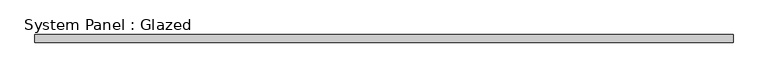
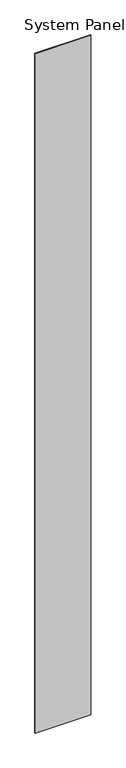
"""IFC4 building model written with IfcOpenShell, lengths in millimetres: plate geometry, System Panel : Glazed."""

from ifc_helpers import new_model, si_unit, origin, origin_with_axes, place, context, project, spatial, polyline, outline, extrude, source, transform, mapped, element, save


def system_panel_glazed_cc704f4b(model_context):
    return source(origin(), model_context, "Body", "SweptSolid", [
        extrude(outline(polyline([(1128.1833333, 19.05), (-1128.1833333, 19.05), (-1128.1833333, 44.45), (1128.1833333, 44.45), (1128.1833333, 19.05)])), origin_with_axes(), (0.0, 0.0, 1.0), 29133.8),
    ])


if __name__ == "__main__":
    model = new_model("IFC4")
    model_context = context("Model", 3, world=origin())
    ifc_project = project(units=[si_unit("LENGTHUNIT", "METRE", prefix="MILLI")], contexts=[model_context])
    site = spatial("IfcSite", under=ifc_project)
    building = spatial("IfcBuilding", under=site)
    placement = place(None, origin())
    system_panel_glazed_shape = system_panel_glazed_cc704f4b(model_context)
    element("IfcPlate", 1, ObjectType="System Panel : Glazed", at=placement, inside=building, context=model_context, shape_type="MappedRepresentation", body=[
        mapped(system_panel_glazed_shape, transform((0.0, 0.0, 0.0), x_axis=(1.0, 0.0, 0.0), y_axis=(0.0, 1.0, 0.0), z_axis=(0.0, 0.0, 1.0))),
    ])
    save(model, "model.ifc")

# Revit data of these elements
# Type "System Panel : Glazed"
#   Construction Type Id = "GSP4R"
#   Analytic Construction = "1/8 in Pilkington single glazing"
#   Visual Light Transmittance = 0.9
#   Solar Heat Gain Coefficient = 0.86
#   Heat Transfer Coefficient (U) = 1.18115 BTU/(h·ft²·°F)
# Element 1 (IfcPlate, "System Panel : Glazed")
#   Materials on its faces: "Glass"
# Materials
#   "Glass": class "Glass", colour RGB 0 128 192, transparency 0.75, Description = "Soda Lime Glass", Cost = 0
